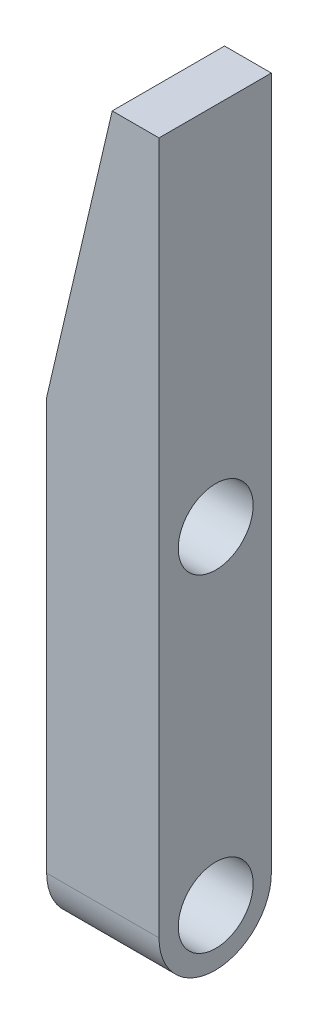
from build123d import *

# Parameters (mm, degrees)
JAW_PLATE_12MM_DEPTH   = 6
ROUNDED_END_SKETCH_R   = 6
ROUNDED_END_BOSS_DEPTH = 12
TAPPED_HOLE_M8X1_25_D  = 8


with BuildPart() as part:
    # Jaw Profile Sketch → Jaw Plate 12mm (new, symmetric)
    with BuildSketch(Plane.XY):
        Polygon((0, 0), (-5, 0), (-12, -30), (-12, -74), (0, -74), align=None)
    extrude(amount=JAW_PLATE_12MM_DEPTH, both=True)

    # Rounded End Sketch → Rounded End Boss (add)
    with BuildSketch(Plane(origin=(0, 0, 0), x_dir=(0, 0, -1), z_dir=(1, 0, 0))):
        with Locations((0, -74)):
            Circle(ROUNDED_END_SKETCH_R)
    extrude(amount=-ROUNDED_END_BOSS_DEPTH)

    # Tapped Hole M8x1.25 (through all)
    with Locations(Plane(origin=(0, -74, -0.055848494), x_dir=(0, 0, 1), z_dir=(1, 0, 0))):
        with Locations((0, 0), (0, -35)):
            Hole(TAPPED_HOLE_M8X1_25_D / 2)


solid = part.part
